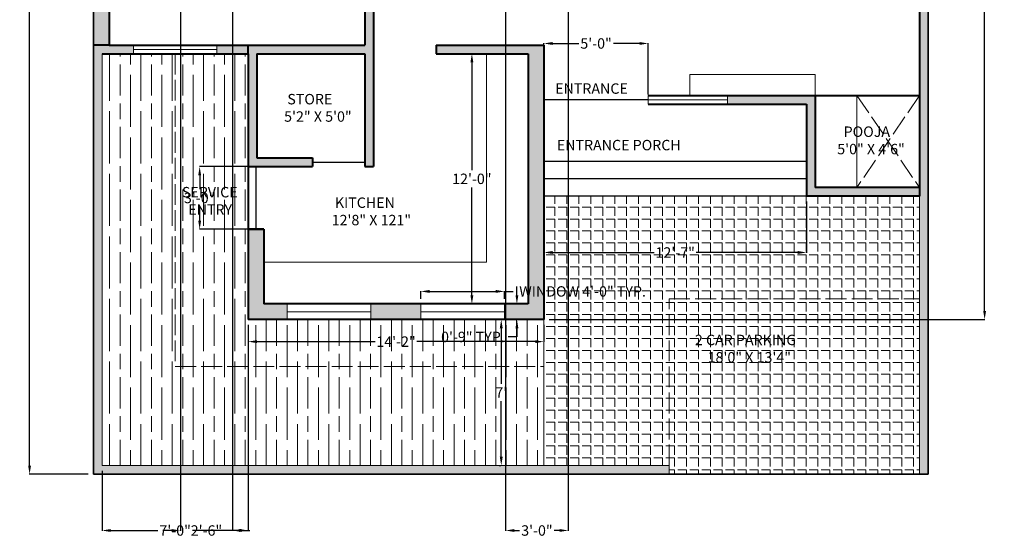
# Model space of a CAD drawing. Units: inches. Extents: x 242 to 808, y 202 to 873.
# Tile 1 of 3: x 242 to 808, y 202 to 500. Entities that reach past the tile are written whole.
import ezdxf

# ---------------------------------------------------------------- set-up
doc = ezdxf.new("R2010")
doc.units = ezdxf.units.IN
doc.header["$MEASUREMENT"] = 0
doc.linetypes.add('ACAD_ISO02W100', pattern=[15, 12, -3])
for name, color, linetype, lineweight in [('A-ANNO-DIMS', 2, 'Continuous', 18), ('A-AREA-IDEN', 7, 'Continuous', 25), ('A-DOOR', 3, 'Continuous', 25), ('A-FLOR-CASE', 8, 'Continuous', 20), ('A-FLOR-CASE-OVHD', 8, 'ACAD_ISO02W100', 13), ('A-FLOR-PATT', 9, 'Continuous', 13), ('A-FLOR-STRS', 7, 'Continuous', 25), ('A-GLAZ', 4, 'Continuous', 18), ('A-ROOF-OVHD', 8, 'ACAD_ISO02W100', 13), ('A-SITE-PVMT', 8, 'Continuous', 18), ('A-SITE-PVMT-PATT', 254, 'Continuous', 13), ('A-WALL', 7, 'Continuous', 40), ('A-WALL-PATT', 30, 'Continuous', 13), ('C-PROP', 7, 'Continuous', 35)]:
    doc.layers.add(name, color=color, linetype=linetype, lineweight=lineweight)
doc.styles.get("Standard").update_dxf_attribs({"font": 'arial.ttf'})
doc.dimstyles.get("Standard").update_dxf_attribs({"dimtxt": 6, "dimasz": 5, "dimexe": 0.18, "dimexo": 3, "dimgap": 2, "dimtad": 0, "dimtih": 1, "dimtoh": 1, "dimdec": 0, "dimzin": 0, "dimdsep": 46, "dimlunit": 3, "dimtxsty": 'Standard', "dimcen": 0.09, "dimadec": 0, "dimazin": 0, "dimtfac": 1, "dimtdec": 0, "dimtofl": 0, "dimtmove": 0, "dimatfit": 3, "dimfxl": 1, "dimtolj": 1, "dimtzin": 0, "dimarcsym": 0})

# ---------------------------------------------------------------- blocks, each defined once
blk = doc.blocks.new('*D3')
at = {"layer": 'A-ANNO-DIMS', "color": 0, "lineweight": -2, "transparency": 16777216}
for p, q in [((373.66, 324.15), (373.66, 314.26)), ((543.66, 324.15), (543.66, 314.26)), ((378.66, 314.44), (446.64, 314.44)), ((538.66, 314.44), (470.69, 314.44))]:
    blk.add_line(p, q, dxfattribs=at)
at = {"layer": 'A-ANNO-DIMS', "color": 0, "transparency": 16777216}
for points in [[(378.66, 315.28), (378.66, 313.61), (373.66, 314.44)], [(538.66, 315.28), (538.66, 313.61), (543.66, 314.44)]]:
    blk.add_solid(points, dxfattribs=at)
at = {"layer": 'Defpoints', "color": 0, "transparency": 16777216}
for p in [(373.66, 327.15), (543.66, 327.15), (543.66, 314.44)]:
    blk.add_point(p, dxfattribs=at)
at = {"layer": 'A-ANNO-DIMS', "color": 0, "transparency": 16777216, "insert": (458.66, 314.44), "char_height": 6, "attachment_point": 5}
blk.add_mtext('\\A1;14\'-2"', dxfattribs=at)
blk = doc.blocks.new('*D4')
at = {"layer": 'A-ANNO-DIMS', "color": 0, "lineweight": -2, "transparency": 16777216}
for p, q in [((517.95, 327.15), (518.97, 327.15)), ((519.15, 322.15), (519.15, 290.15)), ((519.15, 248.15), (519.15, 280.15)), ((517.95, 243.15), (518.97, 243.15))]:
    blk.add_line(p, q, dxfattribs=at)
at = {"layer": 'A-ANNO-DIMS', "color": 0, "transparency": 16777216}
for points in [[(518.32, 322.15), (519.98, 322.15), (519.15, 327.15)], [(518.32, 248.15), (519.98, 248.15), (519.15, 243.15)]]:
    blk.add_solid(points, dxfattribs=at)
at = {"layer": 'Defpoints', "color": 0, "transparency": 16777216}
for p in [(520.95, 327.15), (519.15, 243.15), (520.95, 243.15)]:
    blk.add_point(p, dxfattribs=at)
at = {"layer": 'A-ANNO-DIMS', "color": 0, "transparency": 16777216, "insert": (519.15, 285.15), "char_height": 6, "attachment_point": 5}
blk.add_mtext("\\A1;7'", dxfattribs=at)
blk = doc.blocks.new('*D8')
at = {"layer": 'A-ANNO-DIMS', "color": 0, "lineweight": -2, "transparency": 16777216}
for p, q in [((281.66, 838.15), (247.79, 838.15)), ((247.97, 833.15), (247.97, 543.22)), ((247.97, 243.15), (247.97, 533.09)), ((281.66, 238.15), (247.79, 238.15))]:
    blk.add_line(p, q, dxfattribs=at)
at = {"layer": 'A-ANNO-DIMS', "color": 0, "transparency": 16777216}
for points in [[(247.13, 833.15), (248.8, 833.15), (247.97, 838.15)], [(247.13, 243.15), (248.8, 243.15), (247.97, 238.15)]]:
    blk.add_solid(points, dxfattribs=at)
at = {"layer": 'Defpoints', "color": 0, "transparency": 16777216}
for p in [(284.66, 838.15), (247.97, 238.15), (284.66, 238.15)]:
    blk.add_point(p, dxfattribs=at)
at = {"layer": 'A-ANNO-DIMS', "color": 0, "transparency": 16777216, "insert": (247.97, 538.15), "char_height": 6, "attachment_point": 5}
blk.add_mtext("\\A1;50'", dxfattribs=at)
blk = doc.blocks.new('WIN-48IN')
blk.add_line((4.5, 48), (4.5, 0))
blk.add_lwpolyline([(0, 48), (9, 48), (9, 0), (0, 0)], close=True)
blk = doc.blocks.new('DOOR-30IN-PLAN')
blk.add_line((0, 30), (0, 0))
blk = doc.blocks.new('*D41')
at = {"layer": 'A-ANNO-DIMS', "color": 0, "lineweight": -2, "transparency": 16777216}
for p, q in [((472.95, 339.15), (472.95, 343.53)), ((477.95, 343.35), (515.95, 343.35)), ((520.95, 339.15), (520.95, 343.53)), ((520.95, 343.35), (525.95, 343.35))]:
    blk.add_line(p, q, dxfattribs=at)
at = {"layer": 'A-ANNO-DIMS', "color": 0, "transparency": 16777216}
for points in [[(477.95, 344.19), (477.95, 342.52), (472.95, 343.35)], [(515.95, 344.19), (515.95, 342.52), (520.95, 343.35)]]:
    blk.add_solid(points, dxfattribs=at)
at = {"layer": 'Defpoints', "color": 0, "transparency": 16777216}
for p in [(520.95, 343.35), (472.95, 336.15), (520.95, 336.15)]:
    blk.add_point(p, dxfattribs=at)
at = {"layer": 'A-ANNO-DIMS', "color": 0, "transparency": 16777216, "insert": (565.92, 343.35), "char_height": 6, "attachment_point": 5}
blk.add_mtext('\\A1;WINDOW 4\'-0" TYP.', dxfattribs=at)
blk = doc.blocks.new('*D42')
at = {"layer": 'A-ANNO-DIMS', "color": 0, "lineweight": -2, "transparency": 16777216}
for p, q in [((528.15, 341.15), (528.15, 346.15)), ((523.95, 336.15), (528.33, 336.15)), ((523.95, 327.15), (528.33, 327.15)), ((528.15, 317.15), (523.15, 317.15)), ((528.15, 322.15), (528.15, 317.15))]:
    blk.add_line(p, q, dxfattribs=at)
at = {"layer": 'A-ANNO-DIMS', "color": 0, "transparency": 16777216}
for points in [[(527.32, 341.15), (528.99, 341.15), (528.15, 336.15)], [(527.32, 322.15), (528.99, 322.15), (528.15, 327.15)]]:
    blk.add_solid(points, dxfattribs=at)
at = {"layer": 'Defpoints', "color": 0, "transparency": 16777216}
for p in [(520.95, 336.15), (520.95, 327.15), (528.15, 327.15)]:
    blk.add_point(p, dxfattribs=at)
at = {"layer": 'A-ANNO-DIMS', "color": 0, "transparency": 16777216, "insert": (502.87, 317.15), "char_height": 6, "attachment_point": 5}
blk.add_mtext('\\A1;0\'-9" TYP.', dxfattribs=at)
blk = doc.blocks.new('*D44')
at = {"layer": 'A-ANNO-DIMS', "color": 0, "lineweight": -2, "transparency": 16777216}
for p, q in [((531.66, 480.15), (502.08, 480.15)), ((502.26, 475.15), (502.26, 413.22)), ((502.26, 341.15), (502.26, 403.09)), ((531.66, 336.15), (502.08, 336.15))]:
    blk.add_line(p, q, dxfattribs=at)
at = {"layer": 'A-ANNO-DIMS', "color": 0, "transparency": 16777216}
for points in [[(501.43, 475.15), (503.1, 475.15), (502.26, 480.15)], [(501.43, 341.15), (503.1, 341.15), (502.26, 336.15)]]:
    blk.add_solid(points, dxfattribs=at)
at = {"layer": 'Defpoints', "color": 0, "transparency": 16777216}
for p in [(502.26, 480.15), (534.66, 480.15), (534.66, 336.15)]:
    blk.add_point(p, dxfattribs=at)
at = {"layer": 'A-ANNO-DIMS', "color": 0, "transparency": 16777216, "insert": (502.26, 408.15), "char_height": 6, "attachment_point": 5}
blk.add_mtext('\\A1;12\'-0"', dxfattribs=at)
blk = doc.blocks.new('*D45')
at = {"layer": 'A-ANNO-DIMS', "color": 0, "lineweight": -2, "transparency": 16777216}
for p, q in [((373.66, 324.15), (373.66, 205.57)), ((289.66, 240.15), (289.66, 205.57)), ((294.66, 205.75), (321.71, 205.75)), ((368.66, 205.75), (341.61, 205.75))]:
    blk.add_line(p, q, dxfattribs=at)
at = {"layer": 'A-ANNO-DIMS', "color": 0, "transparency": 16777216}
for points in [[(294.66, 206.59), (294.66, 204.92), (289.66, 205.75)], [(368.66, 206.59), (368.66, 204.92), (373.66, 205.75)]]:
    blk.add_solid(points, dxfattribs=at)
at = {"layer": 'Defpoints', "color": 0, "transparency": 16777216}
for p in [(373.66, 327.15), (289.66, 243.15), (373.66, 205.75)]:
    blk.add_point(p, dxfattribs=at)
at = {"layer": 'A-ANNO-DIMS', "color": 0, "transparency": 16777216, "insert": (331.66, 205.75), "char_height": 6, "attachment_point": 5}
blk.add_mtext('\\A1;7\'-0"', dxfattribs=at)
blk = doc.blocks.new('*D46')
at = {"layer": 'A-ANNO-DIMS', "color": 0, "lineweight": -2, "transparency": 16777216}
for p, q in [((364.66, 626.15), (364.66, 205.57)), ((334.66, 621.65), (334.66, 205.57)), ((329.66, 205.75), (324.66, 205.75)), ((369.66, 205.75), (374.66, 205.75))]:
    blk.add_line(p, q, dxfattribs=at)
at = {"layer": 'A-ANNO-DIMS', "color": 0, "transparency": 16777216}
for points in [[(329.66, 206.59), (329.66, 204.92), (334.66, 205.75)], [(369.66, 206.59), (369.66, 204.92), (364.66, 205.75)]]:
    blk.add_solid(points, dxfattribs=at)
at = {"layer": 'Defpoints', "color": 0, "transparency": 16777216}
for p in [(364.66, 629.15), (334.66, 624.65), (364.66, 205.75)]:
    blk.add_point(p, dxfattribs=at)
at = {"layer": 'A-ANNO-DIMS', "color": 0, "transparency": 16777216, "insert": (349.66, 205.75), "char_height": 6, "attachment_point": 5}
blk.add_mtext('\\A1;2\'-6"', dxfattribs=at)
blk = doc.blocks.new('*D47')
at = {"layer": 'A-ANNO-DIMS', "color": 0, "lineweight": -2, "transparency": 16777216}
for p, q in [((521.66, 617.15), (521.66, 205.57)), ((557.66, 617.15), (557.66, 205.57)), ((526.66, 205.75), (529.69, 205.75)), ((552.66, 205.75), (549.64, 205.75))]:
    blk.add_line(p, q, dxfattribs=at)
at = {"layer": 'A-ANNO-DIMS', "color": 0, "transparency": 16777216}
for points in [[(526.66, 206.59), (526.66, 204.92), (521.66, 205.75)], [(552.66, 206.59), (552.66, 204.92), (557.66, 205.75)]]:
    blk.add_solid(points, dxfattribs=at)
at = {"layer": 'Defpoints', "color": 0, "transparency": 16777216}
for p in [(521.66, 620.15), (557.66, 620.15), (557.66, 205.75)]:
    blk.add_point(p, dxfattribs=at)
at = {"layer": 'A-ANNO-DIMS', "color": 0, "transparency": 16777216, "insert": (539.66, 205.75), "char_height": 6, "attachment_point": 5}
blk.add_mtext('\\A1;3\'-0"', dxfattribs=at)
blk = doc.blocks.new('*D48')
at = {"layer": 'A-ANNO-DIMS', "color": 0, "lineweight": -2, "transparency": 16777216}
for p, q in [((767.66, 838.15), (797.24, 838.15)), ((797.06, 833.15), (797.06, 587.67)), ((797.06, 332.15), (797.06, 577.64)), ((546.66, 327.15), (797.24, 327.15))]:
    blk.add_line(p, q, dxfattribs=at)
at = {"layer": 'A-ANNO-DIMS', "color": 0, "transparency": 16777216}
for points in [[(796.23, 833.15), (797.9, 833.15), (797.06, 838.15)], [(796.23, 332.15), (797.9, 332.15), (797.06, 327.15)]]:
    blk.add_solid(points, dxfattribs=at)
at = {"layer": 'Defpoints', "color": 0, "transparency": 16777216}
for p in [(764.66, 838.15), (797.06, 838.15), (543.66, 327.15)]:
    blk.add_point(p, dxfattribs=at)
at = {"layer": 'A-ANNO-DIMS', "color": 0, "transparency": 16777216, "insert": (797.06, 582.65), "char_height": 6, "attachment_point": 5}
blk.add_mtext('\\A1;42\'-7"', dxfattribs=at)
blk = doc.blocks.new('*D53')
at = {"layer": 'A-ANNO-DIMS', "color": 0, "lineweight": -2, "transparency": 16777216}
for p, q in [((543.66, 456.65), (543.66, 486.23)), ((548.66, 486.05), (563.69, 486.05)), ((598.66, 486.05), (583.64, 486.05)), ((603.66, 456.65), (603.66, 486.23))]:
    blk.add_line(p, q, dxfattribs=at)
at = {"layer": 'A-ANNO-DIMS', "color": 0, "transparency": 16777216}
for points in [[(548.66, 486.89), (548.66, 485.22), (543.66, 486.05)], [(598.66, 486.89), (598.66, 485.22), (603.66, 486.05)]]:
    blk.add_solid(points, dxfattribs=at)
at = {"layer": 'Defpoints', "color": 0, "transparency": 16777216}
for p in [(603.66, 486.05), (543.66, 453.65), (603.66, 453.65)]:
    blk.add_point(p, dxfattribs=at)
at = {"layer": 'A-ANNO-DIMS', "color": 0, "transparency": 16777216, "insert": (573.66, 486.05), "char_height": 6, "attachment_point": 5}
blk.add_mtext('\\A1;5\'-0"', dxfattribs=at)
blk = doc.blocks.new('*D54')
at = {"layer": 'A-ANNO-DIMS', "color": 0, "lineweight": -2, "transparency": 16777216}
for p, q in [((543.66, 395.15), (543.66, 365.57)), ((694.66, 395.15), (694.66, 365.57)), ((548.66, 365.75), (607.14, 365.75)), ((689.66, 365.75), (631.19, 365.75))]:
    blk.add_line(p, q, dxfattribs=at)
at = {"layer": 'A-ANNO-DIMS', "color": 0, "transparency": 16777216}
for points in [[(548.66, 366.59), (548.66, 364.92), (543.66, 365.75)], [(689.66, 366.59), (689.66, 364.92), (694.66, 365.75)]]:
    blk.add_solid(points, dxfattribs=at)
at = {"layer": 'Defpoints', "color": 0, "transparency": 16777216}
for p in [(543.66, 398.15), (694.66, 398.15), (543.66, 365.75)]:
    blk.add_point(p, dxfattribs=at)
at = {"layer": 'A-ANNO-DIMS', "color": 0, "transparency": 16777216, "insert": (619.16, 365.75), "char_height": 6, "attachment_point": 5}
blk.add_mtext('\\A1;12\'-7"', dxfattribs=at)
blk = doc.blocks.new('*D55')
at = {"layer": 'A-ANNO-DIMS', "color": 0, "lineweight": -2, "transparency": 16777216}
for p, q in [((375.16, 415.15), (345.58, 415.15)), ((345.76, 410.15), (345.76, 402.22)), ((345.76, 384.15), (345.76, 392.09)), ((375.16, 379.15), (345.58, 379.15))]:
    blk.add_line(p, q, dxfattribs=at)
at = {"layer": 'A-ANNO-DIMS', "color": 0, "transparency": 16777216}
for points in [[(344.93, 410.15), (346.6, 410.15), (345.76, 415.15)], [(344.93, 384.15), (346.6, 384.15), (345.76, 379.15)]]:
    blk.add_solid(points, dxfattribs=at)
at = {"layer": 'Defpoints', "color": 0, "transparency": 16777216}
for p in [(345.76, 415.15), (378.16, 415.15), (378.16, 379.15)]:
    blk.add_point(p, dxfattribs=at)
at = {"layer": 'A-ANNO-DIMS', "color": 0, "transparency": 16777216, "insert": (345.76, 397.15), "char_height": 6, "attachment_point": 5}
blk.add_mtext('\\A1;3\'-0"', dxfattribs=at)

msp = doc.modelspace()

# ---------------------------------------------------------------- hatches: boundary and pattern name
at = {"layer": 'A-FLOR-PATT'}
h = msp.add_hatch(dxfattribs=at)
h.set_pattern_fill('GOST_WOOD', color=256, scale=3, angle=180)
h.set_pattern_definition([(270, (0, 0), (-18, 3e-15), [30, -6]), (270, (-6, 6), (-18, 3e-15), [18, -4.5, 9, -4.5]), (270, (-12, 15), (-18, 3e-15), [30, -6])])
h.paths.add_polyline_path([(331.66, 480.15), (289.66, 480.15), (289.66, 243.15), (543.66, 243.15), (543.66, 300.15), (331.66, 300.15)])
h.paths.add_polyline_path([(373.66, 480.15), (331.66, 480.15), (331.66, 300.15), (543.66, 300.15), (543.66, 327.15), (373.66, 327.15)], flags=17)
h.paths.add_polyline_path([(333.66, 384.1), (373.46, 384.1), (373.46, 406.46), (333.66, 406.46)], flags=24)
at = {"layer": 'A-SITE-PVMT-PATT'}
h = msp.add_hatch(dxfattribs=at)
h.set_pattern_fill('ANGLE', color=256, scale=25, angle=180)
h.set_pattern_definition([(180, (0, 0), (-8e-16, -6.875), [5, -1.875]), (270, (0, 0), (6.875, -1e-15), [5, -1.875])])
h.paths.add_polyline_path([(759.66, 398.15), (694.66, 398.15), (543.66, 398.15), (543.66, 327.15), (543.66, 243.15), (615.66, 243.15), (615.66, 339.15), (759.66, 339.15)])
h.paths.add_polyline_path([(759.66, 339.15), (615.66, 339.15), (615.66, 243.15), (615.66, 238.15), (759.66, 238.15)])
h.paths.add_polyline_path([(628.74, 299.01), (696.48, 299.01), (696.48, 321.4), (628.74, 321.4)], flags=24)
at = {"layer": 'A-WALL-PATT'}
h = msp.add_hatch(color=256, dxfattribs=at)
h.dxf.hatch_style = 1
h.paths.add_polyline_path([(521.66, 838.15), (325.66, 838.15), (325.66, 789.05), (334.66, 789.05), (334.66, 829.15), (512.66, 829.15), (512.66, 788.15), (714.66, 788.15), (723.66, 788.15), (723.66, 797.15), (521.66, 797.15)])
h.paths.add_polyline_path([(764.66, 838.15), (521.66, 838.15), (521.66, 833.15), (759.66, 833.15), (759.66, 629.15), (764.66, 629.15)])
h.paths.add_polyline_path([(723.66, 788.15), (714.66, 788.15), (714.66, 767.17), (723.66, 767.17)], flags=17)
h.paths.add_polyline_path([(723.66, 743.17), (714.66, 743.17), (714.66, 721.15), (622.66, 721.15), (622.66, 758.15), (617.66, 758.15), (617.66, 721.15), (521.66, 721.15), (521.66, 716.15), (643.66, 716.15), (643.66, 659.15), (648.66, 659.15), (648.66, 716.15), (714.66, 716.15), (714.66, 688.28), (723.66, 688.28)], flags=17)
h.paths.add_polyline_path([(764.66, 629.15), (759.66, 629.15), (723.66, 629.15), (723.66, 664.28), (714.66, 664.28), (714.66, 629.15), (648.66, 629.15), (643.66, 629.15), (643.66, 620.15), (759.66, 620.15), (759.66, 403.15), (759.66, 398.15), (759.66, 238.15), (764.66, 238.15)])
h.paths.add_polyline_path([(521.66, 758.15), (512.66, 758.15), (512.66, 620.15), (521.66, 620.15)])
h.paths.add_polyline_path([(481.66, 694.15), (334.66, 694.15), (334.66, 689.15), (476.66, 689.15), (476.66, 629.15), (481.66, 629.15)])
h.paths.add_polyline_path([(334.66, 741.05), (325.66, 741.05), (325.66, 675.31), (334.66, 675.31), (334.66, 689.15), (334.66, 694.15)], flags=17)
h.paths.add_polyline_path([(334.66, 651.31), (325.66, 651.31), (325.66, 629.15), (289.66, 629.15), (289.66, 838.15), (284.66, 838.15), (284.66, 620.15), (293.66, 620.15), (334.66, 620.15)])
h.paths.add_polyline_path([(293.66, 620.15), (284.66, 620.15), (284.66, 485.15), (293.66, 485.15)])
h.paths.add_polyline_path([(307.66, 485.15), (293.66, 485.15), (284.66, 485.15), (284.66, 238.15), (615.66, 238.15), (615.66, 243.15), (289.66, 243.15), (289.66, 480.15), (307.66, 480.15)])
h.paths.add_polyline_path([(373.66, 485.15), (355.66, 485.15), (355.66, 480.15), (373.66, 480.15)], flags=17)
h.paths.add_polyline_path([(445.66, 620.15), (440.66, 620.15), (440.66, 485.15), (373.66, 485.15), (373.66, 480.15), (373.66, 415.15), (410.66, 415.15), (410.66, 420.15), (378.66, 420.15), (378.66, 480.15), (440.66, 480.15), (440.66, 415.15), (445.66, 415.15)])
h.paths.add_polyline_path([(472.95, 336.15), (444.15, 336.15), (444.15, 327.15), (472.95, 327.15)], flags=17)
h.paths.add_polyline_path([(543.66, 485.15), (481.66, 485.15), (481.66, 480.15), (534.66, 480.15), (534.66, 336.15), (520.95, 336.15), (520.95, 327.15), (543.66, 327.15)], flags=17)
h.paths.add_polyline_path([(699.66, 456.15), (649.16, 456.15), (649.16, 451.15), (694.66, 451.15), (694.66, 398.15), (759.66, 398.15), (759.66, 403.15), (699.66, 403.15)], flags=17)
h.paths.add_polyline_path([(481.66, 629.15), (476.66, 629.15), (364.66, 629.15), (364.66, 620.15), (481.66, 620.15)])
h = msp.add_hatch(color=256, dxfattribs=at)
h.dxf.hatch_style = 1
h.paths.add_polyline_path([(382.66, 379.15), (373.66, 379.15), (373.66, 327.15), (396.15, 327.15), (396.15, 336.15), (382.66, 336.15)])

# ---------------------------------------------------------------- linework, layer by layer
at = {"layer": 'A-DOOR'}
for p, q in [((603.66, 453.65), (543.66, 453.65)), ((378.16, 379.15), (378.16, 415.15))]:
    msp.add_line(p, q, dxfattribs=at)
at = {"layer": 'A-FLOR-CASE'}
for p, q in [((510.66, 480.15), (510.66, 360.15)), ((699.66, 468.15), (627.66, 468.15)), ((627.66, 468.15), (627.66, 456.15)), ((699.66, 456.15), (699.66, 468.15)), ((723.66, 456.15), (723.66, 403.15)), ((510.66, 360.15), (382.66, 360.15))]:
    msp.add_line(p, q, dxfattribs=at)
at = {"layer": 'A-FLOR-CASE-OVHD'}
for p, q in [((759.66, 456.15), (723.66, 403.15)), ((723.66, 456.15), (759.66, 403.15))]:
    msp.add_line(p, q, dxfattribs=at)
at = {"layer": 'A-FLOR-STRS'}
for p, q in [((694.66, 418.15), (543.66, 418.15)), ((694.66, 408.15), (543.66, 408.15)), ((694.66, 398.15), (543.66, 398.15))]:
    msp.add_line(p, q, dxfattribs=at)
at = {"layer": 'A-GLAZ'}
for p, q in [((307.66, 480.15), (307.66, 485.15)), ((307.66, 482.65), (355.66, 482.65)), ((355.66, 480.15), (355.66, 485.15)), ((603.66, 456.15), (603.66, 451.15)), ((649.16, 453.65), (603.66, 453.65)), ((649.16, 451.15), (649.16, 456.15))]:
    msp.add_line(p, q, dxfattribs=at)
at = {"layer": 'A-ROOF-OVHD'}
for p, q in [((331.66, 480.15), (331.66, 300.15)), ((615.66, 243.15), (615.66, 339.15)), ((615.66, 339.15), (759.66, 339.15)), ((331.66, 300.15), (543.66, 300.15))]:
    msp.add_line(p, q, dxfattribs=at)
at = {"layer": 'A-SITE-PVMT'}
for p, q in [((289.66, 480.15), (289.66, 243.15)), ((759.66, 398.15), (759.66, 238.15)), ((543.66, 327.15), (543.66, 243.15)), ((615.66, 243.15), (289.66, 243.15)), ((615.66, 243.15), (615.66, 238.15))]:
    msp.add_line(p, q, dxfattribs=at)
at = {"layer": 'A-WALL'}
for p, q in [((293.66, 620.15), (293.66, 485.15)), ((440.66, 620.15), (440.66, 485.15)), ((445.66, 620.15), (445.66, 415.15)), ((759.66, 620.15), (759.66, 403.15)), ((293.66, 485.15), (284.66, 485.15)), ((293.66, 485.15), (440.66, 485.15)), ((373.66, 480.15), (373.66, 485.15)), ((481.66, 485.15), (481.66, 480.15)), ((481.66, 485.15), (543.66, 485.15)), ((543.66, 485.15), (543.66, 327.15)), ((289.66, 480.15), (373.66, 480.15)), ((373.66, 480.15), (373.66, 327.15)), ((378.66, 480.15), (378.66, 420.15)), ((378.66, 480.15), (440.66, 480.15)), ((440.66, 480.15), (440.66, 415.15)), ((481.66, 480.15), (534.66, 480.15)), ((534.66, 480.15), (534.66, 336.15)), ((603.66, 456.15), (759.66, 456.15)), ((699.66, 456.15), (699.66, 403.15)), ((603.66, 451.15), (694.66, 451.15)), ((694.66, 451.15), (694.66, 398.15)), ((378.66, 420.15), (410.66, 420.15)), ((410.66, 420.15), (410.66, 415.15)), ((373.66, 415.15), (410.66, 415.15)), ((440.66, 415.15), (445.66, 415.15)), ((759.66, 403.15), (699.66, 403.15)), ((759.66, 403.15), (759.66, 398.15)), ((759.66, 398.15), (694.66, 398.15)), ((373.66, 379.15), (382.66, 379.15)), ((382.66, 379.15), (373.66, 379.15)), ((382.66, 379.15), (373.66, 379.15)), ((382.66, 379.15), (382.66, 336.15)), ((534.66, 336.15), (382.66, 336.15)), ((543.66, 327.15), (373.66, 327.15))]:
    msp.add_line(p, q, dxfattribs=at)
at = {"layer": 'C-PROP'}
for p, q in [((284.66, 238.15), (284.66, 838.15)), ((764.66, 838.15), (764.66, 238.15)), ((764.66, 238.15), (284.66, 238.15))]:
    msp.add_line(p, q, dxfattribs=at)

# ---------------------------------------------------------------- block references
at = {"layer": 'A-DOOR', "rotation": 90}
msp.add_blockref('DOOR-30IN-PLAN', (440.66, 417.65), dxfattribs=at)
at = {"layer": 'A-GLAZ', "rotation": 269.9999999999998}
for p in [(396.15, 336.15), (472.95, 336.15)]:
    msp.add_blockref('WIN-48IN', p, dxfattribs=at)

# ---------------------------------------------------------------- texts
at = {"layer": 'A-AREA-IDEN', "char_height": 6, "attachment_point": 1}
for s, heights, insert in [('ENTRANCE', [0], (550.14, 463.09)), (' STORE\\P5\'2" X 5\'0"', [0], (394.32, 457)), ('  POOJA \\P5\'0" X 4\'6"', [0], (712.33, 438.29)), ('ENTRANCE PORCH', [0], (551.1, 430.56)), ('SERVICE\\P  ENTRY', [0], (335.54, 403.47)), (' KITCHEN\\P12\'8" X 121"', [16.23], (421.66, 397.41)), ('2 CAR PARKING \\P    18\'0" X 13\'4"', [0], (630.48, 318.41))]:
    msp.add_mtext_dynamic_manual_height_columns(s, width=78.0144, gutter_width=1, heights=heights, dxfattribs=dict(at, insert=insert))

# ---------------------------------------------------------------- dimensions: what is measured, and where the dimension line sits
at = {"layer": 'A-ANNO-DIMS'}
for base, p1, p2, angle, override, picture, middle in [((247.97, 238.15), (284.66, 838.15), (284.66, 238.15), 90, {"dimclrd": 0, "dimclre": 0, "dimclrt": 0}, '*D8', (247.97, 538.15)), ((797.06, 838.15), (543.66, 327.15), (764.66, 838.15), 90, {"dimdec": 1, "dimlfac": 1, "dimrnd": 0, "dimzin": 1, "dimdsep": 46, "dimlunit": 4, "dimfrac": 2}, '*D48', (797.06, 582.65)), ((502.26, 480.15), (534.66, 336.15), (534.66, 480.15), 90, {"dimdec": 1, "dimlfac": 1, "dimrnd": 0, "dimzin": 1, "dimdsep": 46, "dimlunit": 4, "dimfrac": 2}, '*D44', (502.26, 408.15)), ((345.76, 415.15), (378.16, 379.15), (378.16, 415.15), 90, {"dimdec": 1, "dimlfac": 1, "dimrnd": 0, "dimzin": 1, "dimdsep": 46, "dimlunit": 4, "dimfrac": 2}, '*D55', (345.76, 397.15)), ((543.66, 365.75), (694.66, 398.15), (543.66, 398.15), 180, {"dimdec": 1, "dimlfac": 1, "dimrnd": 0, "dimzin": 1, "dimdsep": 46, "dimlunit": 4, "dimfrac": 2}, '*D54', (619.16, 365.75)), ((519.15, 243.15), (520.95, 327.15), (520.95, 243.15), 90, {"dimclrd": 0, "dimclre": 0, "dimclrt": 0}, '*D4', (519.15, 285.15))]:
    dim = msp.add_linear_dim(base=base, p1=p1, p2=p2, angle=angle, dimstyle='Standard', override=override, dxfattribs=at)
    dim.commit()
    dim.dimension.update_dxf_attribs({"geometry": picture, "text_midpoint": middle})
for base, p1, p2, override, picture, middle in [((364.66, 205.75), (334.66, 624.65), (364.66, 629.15), {"dimdec": 1, "dimlfac": 1, "dimrnd": 0, "dimzin": 1, "dimdsep": 46, "dimlunit": 4, "dimfrac": 2}, '*D46', (349.66, 205.75)), ((557.66, 205.75), (521.66, 620.15), (557.66, 620.15), {"dimdec": 1, "dimlfac": 1, "dimrnd": 0, "dimzin": 1, "dimdsep": 46, "dimlunit": 4, "dimfrac": 2}, '*D47', (539.66, 205.75)), ((603.66, 486.05), (543.66, 453.65), (603.66, 453.65), {"dimdec": 1, "dimlfac": 1, "dimrnd": 0, "dimzin": 1, "dimdsep": 46, "dimlunit": 4, "dimfrac": 2}, '*D53', (573.66, 486.05)), ((373.66, 205.75), (289.66, 243.15), (373.66, 327.15), {"dimdec": 1, "dimlfac": 1, "dimrnd": 0, "dimzin": 1, "dimdsep": 46, "dimlunit": 4, "dimfrac": 2}, '*D45', (331.66, 205.75)), ((543.66, 314.44), (373.66, 327.15), (543.66, 327.15), {"dimclrd": 0, "dimclre": 0, "dimclrt": 0}, '*D3', (458.66, 314.44))]:
    dim = msp.add_linear_dim(base=base, p1=p1, p2=p2, dimstyle='Standard', override=override, dxfattribs=at)
    dim.commit()
    dim.dimension.update_dxf_attribs({"geometry": picture, "text_midpoint": middle})
dim = msp.add_linear_dim(base=(520.95, 343.35), p1=(472.95, 336.15), p2=(520.95, 336.15), text='WINDOW <> TYP.', dimstyle='Standard', override={"dimdec": 1, "dimlfac": 1, "dimrnd": 0, "dimzin": 1, "dimdsep": 46, "dimlunit": 4, "dimfrac": 2}, dxfattribs=at)
dim.commit()
dim.dimension.update_dxf_attribs({"geometry": '*D41', "text_midpoint": (565.92, 343.35)})
dim = msp.add_linear_dim(base=(528.15, 327.15), p1=(520.95, 336.15), p2=(520.95, 327.15), angle=270, text='<> TYP.', dimstyle='Standard', override={"dimdec": 1, "dimlfac": 1, "dimrnd": 0, "dimzin": 1, "dimdsep": 46, "dimlunit": 4, "dimfrac": 2}, dxfattribs=at)
dim.commit()
dim.dimension.update_dxf_attribs({"geometry": '*D42', "text_midpoint": (502.87, 317.15)})

doc.saveas('drawing.dxf')
